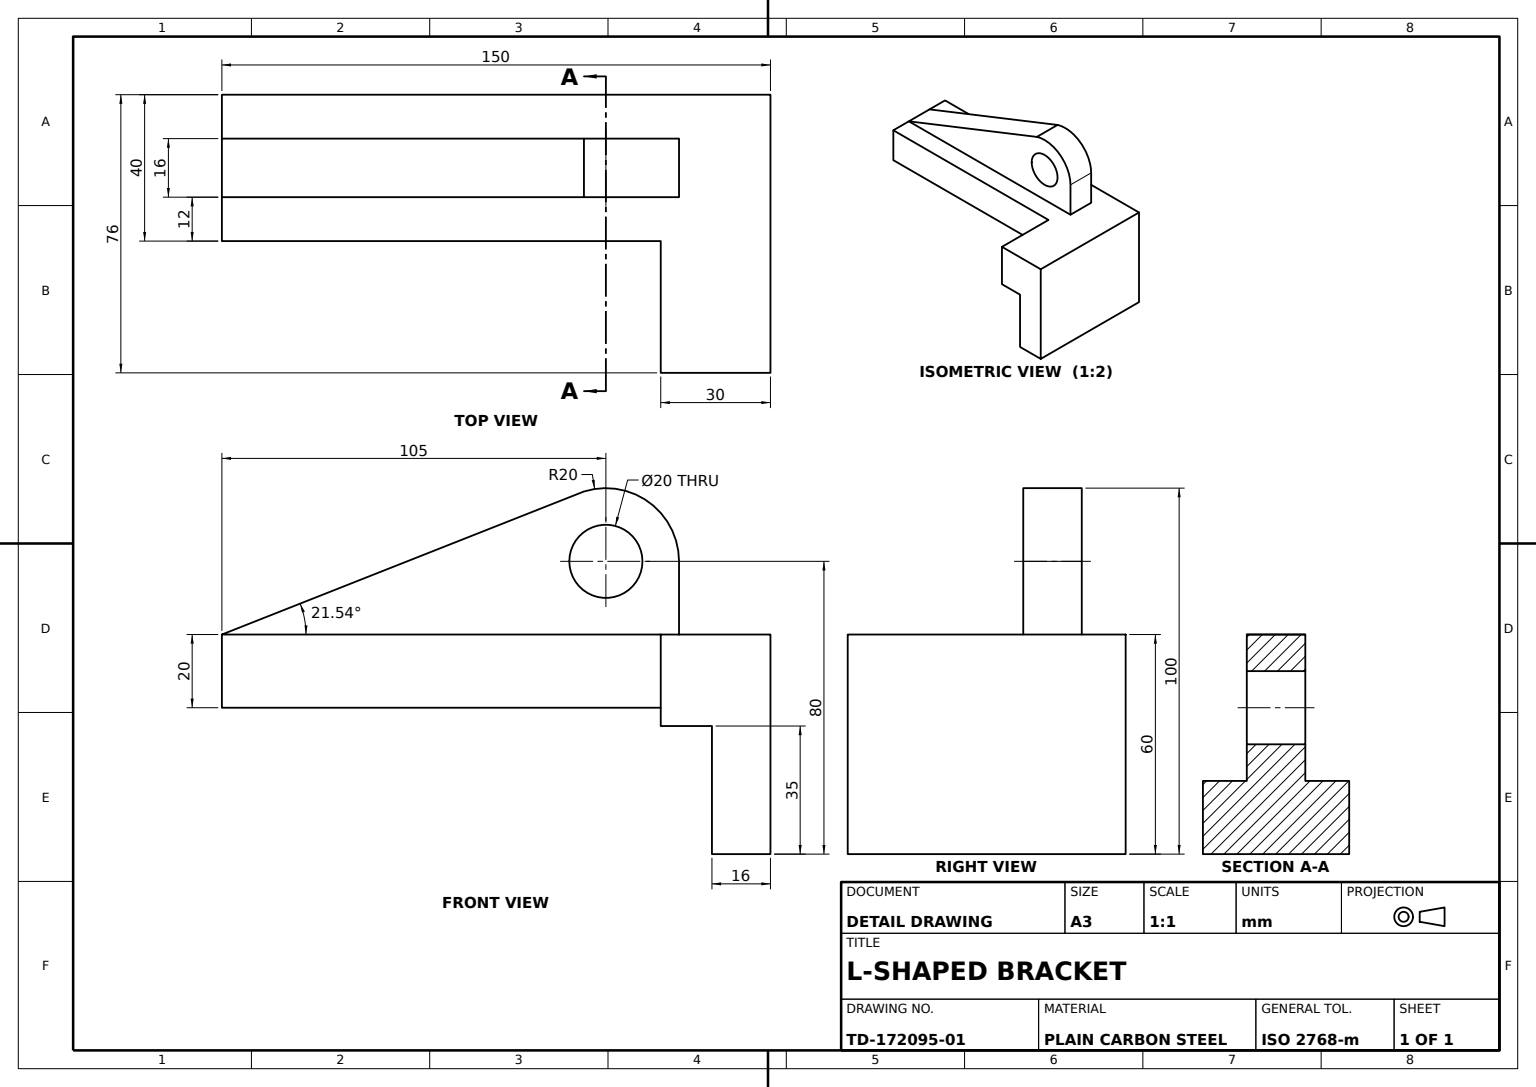
from build123d import *

# Parameters (mm, degrees)
BASE_PLATE_SKETCH_W    = 76
BASE_PLATE_SKETCH_H    = 60
BASE_PLATE_DEPTH       = 16
UPRIGHT_WALL_DEPTH     = 76
WALL_NOTCH_SKETCH_W    = 76
WALL_NOTCH_SKETCH_H    = 25
WALL_NOTCH_DEPTH       = 16
ARM_BLOCK_SKETCH_W     = 120
ARM_BLOCK_SKETCH_H     = 20
ARM_BLOCK_DEPTH        = 40
ARM_LUG_DEPTH          = 40
ARM_SIDE_CUT_A_DEPTH   = 12
ARM_START              = -12
ARM_SIDE_CUT_B_DEPTH   = 12
PIVOT_HOLE_20_SKETCH_R = 10
PIVOT_HOLE_20_DEPTH    = 16


with BuildPart() as part:
    # Base Plate Sketch → Base Plate (new body)
    with BuildSketch(Plane.XY):
        with Locations((38, 30)):
            Rectangle(BASE_PLATE_SKETCH_W, BASE_PLATE_SKETCH_H)
    extrude(amount=BASE_PLATE_DEPTH)

    # Upright Wall Sketch → Upright Wall (add)
    with BuildSketch(Plane(origin=(76, 0, 0), x_dir=(0, 0, -1), z_dir=(1, 0, 0))):
        Polygon((-16, 60), (-41, 60), (-46, 60), (-46, 35), (-16, 35), align=None)
    extrude(amount=-UPRIGHT_WALL_DEPTH)

    # Wall Notch Sketch → Wall Notch (cut)
    with BuildSketch(Plane.XY.offset(46)):
        with Locations((38, 47.5)):
            Rectangle(WALL_NOTCH_SKETCH_W, WALL_NOTCH_SKETCH_H)
    extrude(amount=-WALL_NOTCH_DEPTH, mode=Mode.SUBTRACT)

    # Arm Block Sketch → Arm Block (add)
    with BuildSketch(Plane.ZY):
        with Locations((90, 50)):
            Rectangle(ARM_BLOCK_SKETCH_W, ARM_BLOCK_SKETCH_H)
    extrude(amount=-ARM_BLOCK_DEPTH)

    # Arm Lug Sketch → Arm Lug (add)
    with BuildSketch(Plane(origin=(40, 0, 0), x_dir=(0, 0, -1), z_dir=(1, 0, 0))):
        with BuildLine():
            Line((-53.649750889, 98.032798162), (-150, 60))
            Line((-150, 60), (-30, 60))
            Line((-30, 60), (-25, 60))
            Line((-25, 60), (-25, 80))
            ThreePointArc((-25, 80), (-33.167646012, 96.124372828), (-50.99953991, 99.078928714))
            Line((-50.99953991, 99.078928714), (-53.649750889, 98.032798162))
        make_face()
    extrude(amount=-ARM_LUG_DEPTH)

    # Arm Side Cut A Sketch → Arm Side Cut A (cut)
    with BuildSketch(Plane(origin=(40, 0, 0), x_dir=(0, 0, -1), z_dir=(1, 0, 0))):
        with BuildLine():
            Line((-53.649750889, 98.032798162), (-150, 60))
            Line((-150, 60), (-30, 60))
            Line((-30, 60), (-25, 60))
            Line((-25, 60), (-25, 80))
            ThreePointArc((-25, 80), (-33.167646012, 96.124372828), (-50.99953991, 99.078928714))
            Line((-50.99953991, 99.078928714), (-53.649750889, 98.032798162))
        make_face()
    extrude(amount=-ARM_SIDE_CUT_A_DEPTH, mode=Mode.SUBTRACT)

    # Arm Side Cut B Sketch → Arm Side Cut B (cut)
    with BuildSketch(Plane.ZY.offset(ARM_START)):
        with BuildLine():
            Line((25, 80), (25, 60))
            Line((25, 60), (150, 60))
            Line((150, 60), (53.649750889, 98.032798162))
            Line((53.649750889, 98.032798162), (50.99953991, 99.078928714))
            ThreePointArc((50.99953991, 99.078928714), (33.167646012, 96.124372828), (25, 80))
        make_face()
    extrude(amount=ARM_SIDE_CUT_B_DEPTH, mode=Mode.SUBTRACT)

    # Pivot Hole Ø20 Sketch → Pivot Hole Ø20 (cut)
    with BuildSketch(Plane(origin=(28, 0, 0), x_dir=(0, 0, -1), z_dir=(1, 0, 0))):
        with Locations((-45, 80)):
            Circle(PIVOT_HOLE_20_SKETCH_R)
    extrude(amount=-PIVOT_HOLE_20_DEPTH, mode=Mode.SUBTRACT)


solid = part.part
